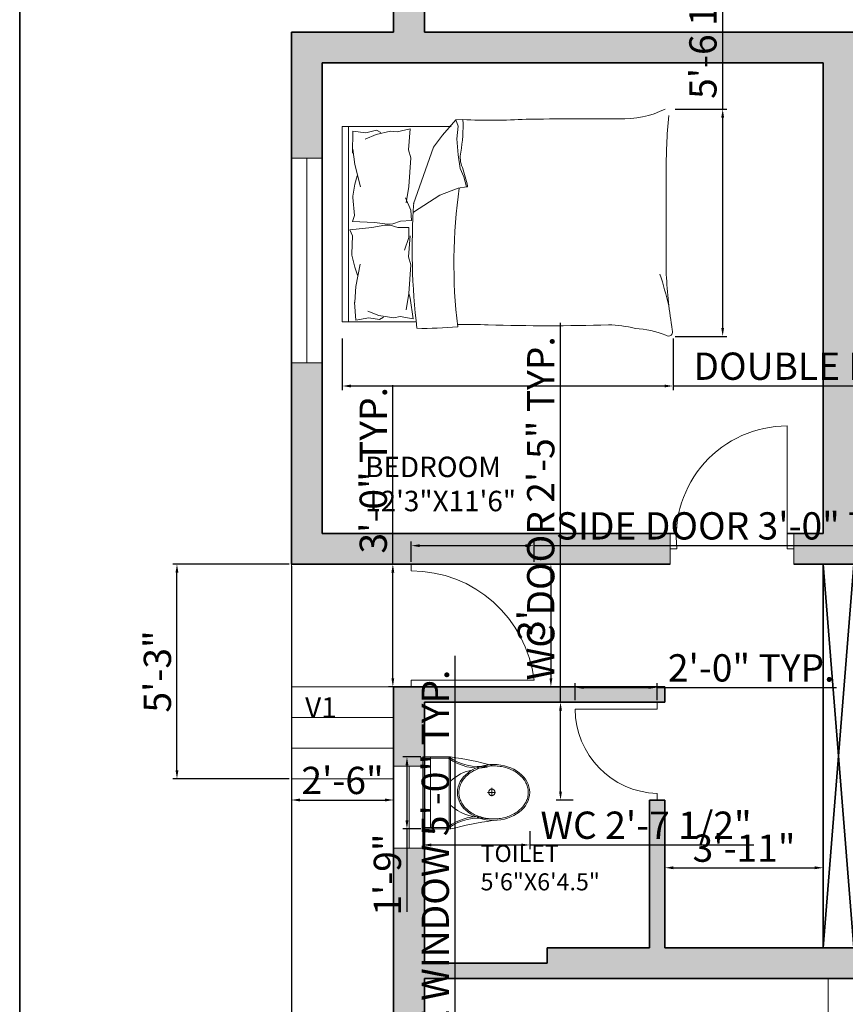
# Model space of a CAD drawing. Units: inches. Extents: x 2257 to 3678, y 834 to 1975.
# Tile 2 of 16: x 2257 to 2500, y 1155 to 1444. Entities that reach past the tile are written whole.
import ezdxf

# ---------------------------------------------------------------- set-up
doc = ezdxf.new("R2010")
doc.units = ezdxf.units.IN
for name, color, linetype, lineweight in [('A-ANNO-DIMS', 2, 'Continuous', 18), ('A-ANNO-TEXT', 7, 'Continuous', 18), ('A-ANNO-TTLB', 7, 'Continuous', 35), ('A-AREA-IDEN', 7, 'Continuous', 18), ('A-DOOR', 3, 'Continuous', 18), ('A-FLOR-CASE', 8, 'Continuous', 18), ('A-FLOR-FIXT', 9, 'Continuous', 18), ('A-FLOR-STRS', 7, 'Continuous', 18), ('A-FURN', 8, 'Continuous', 18), ('A-GLAZ', 4, 'Continuous', 18), ('A-WALL', 7, 'Continuous', 35)]:
    doc.layers.add(name, color=color, linetype=linetype, lineweight=lineweight)
doc.layers.add('A-WALL-PATT', color=251, linetype='Continuous', lineweight=13, true_color=0x636466)
doc.styles.get("Standard").update_dxf_attribs({"font": 'arial.ttf'})
doc.dimstyles.new('ISO-25', dxfattribs={"dimtxt": 8, "dimasz": 2.5, "dimexe": 1.25, "dimexo": 0.625, "dimtad": 1, "dimdec": 0, "dimlunit": 3, "dimtxsty": 'Standard', "dimcen": 2.5, "dimadec": 0, "dimazin": 0, "dimtfac": 1, "dimtdec": 0, "dimtmove": 0, "dimatfit": 3, "dimfxl": 1, "dimarcsym": 0})

# ---------------------------------------------------------------- blocks, each defined once
blk = doc.blocks.new('*D4')
at = {"layer": 'A-ANNO-DIMS', "color": 0, "lineweight": -2, "transparency": 16777216}
for p, q in [((2407.1, 1284.58), (2414.41, 1284.58)), ((2413.16, 1282.08), (2413.16, 1251.08)), ((2407.1, 1248.58), (2414.41, 1248.58))]:
    blk.add_line(p, q, dxfattribs=at)
at = {"layer": 'A-ANNO-DIMS', "color": 0, "transparency": 16777216}
for points in [[(2412.75, 1282.08), (2413.58, 1282.08), (2413.16, 1284.58)], [(2412.75, 1251.08), (2413.58, 1251.08), (2413.16, 1248.58)]]:
    blk.add_solid(points, dxfattribs=at)
at = {"layer": 'Defpoints', "color": 0, "transparency": 16777216}
for p in [(2406.47, 1284.58), (2406.47, 1248.58), (2413.16, 1248.58)]:
    blk.add_point(p, dxfattribs=at)
at = {"layer": 'A-ANNO-DIMS', "color": 0, "transparency": 16777216, "insert": (2408.45, 1266.58), "char_height": 8, "attachment_point": 5, "rotation": 90}
blk.add_mtext("3'", dxfattribs=at)
blk = doc.blocks.new('*D5')
at = {"layer": 'A-ANNO-DIMS', "color": 0, "lineweight": -2, "transparency": 16777216}
for p, q in [((2446.55, 1196.14), (2446.55, 1196.77)), ((2449.05, 1195.52), (2490.55, 1195.52)), ((2493.05, 1196.14), (2493.05, 1196.77))]:
    blk.add_line(p, q, dxfattribs=at)
at = {"layer": 'A-ANNO-DIMS', "color": 0, "transparency": 16777216}
for points in [[(2449.05, 1195.94), (2449.05, 1195.1), (2446.55, 1195.52)], [(2490.55, 1195.94), (2490.55, 1195.1), (2493.05, 1195.52)]]:
    blk.add_solid(points, dxfattribs=at)
at = {"layer": 'Defpoints', "color": 0, "transparency": 16777216}
for p in [(2446.55, 1195.52), (2493.05, 1195.52), (2493.05, 1195.52)]:
    blk.add_point(p, dxfattribs=at)
at = {"layer": 'A-ANNO-DIMS', "color": 0, "transparency": 16777216, "insert": (2469.8, 1200.23), "char_height": 8, "attachment_point": 5}
blk.add_mtext('3\'-11"', dxfattribs=at)
blk = doc.blocks.new('*D6')
at = {"layer": 'A-ANNO-DIMS', "color": 0, "lineweight": -2, "transparency": 16777216}
for p, q in [((2337.05, 1220.95), (2337.05, 1214.14)), ((2367.05, 1220.95), (2367.05, 1214.14)), ((2339.55, 1215.39), (2364.55, 1215.39))]:
    blk.add_line(p, q, dxfattribs=at)
at = {"layer": 'A-ANNO-DIMS', "color": 0, "transparency": 16777216}
for points in [[(2339.55, 1215.8), (2339.55, 1214.97), (2337.05, 1215.39)], [(2364.55, 1215.8), (2364.55, 1214.97), (2367.05, 1215.39)]]:
    blk.add_solid(points, dxfattribs=at)
at = {"layer": 'Defpoints', "color": 0, "transparency": 16777216}
for p in [(2337.05, 1221.58), (2367.05, 1221.58), (2367.05, 1215.39)]:
    blk.add_point(p, dxfattribs=at)
at = {"layer": 'A-ANNO-DIMS', "color": 0, "transparency": 16777216, "insert": (2352.05, 1220.09), "char_height": 8, "attachment_point": 5}
blk.add_mtext('2\'-6"', dxfattribs=at)
blk = doc.blocks.new('A$C31115884')
for p, q in [((283.1, 497.7), (223.4, 497.7)), ((257.5, 466.4), (257.5, 523.2)), ((0, 200), (0, 0)), ((520, 200), (0, 200)), ((10, 190), (10, 10)), ((510, 190), (10, 190)), ((510, 10), (510, 190)), ((520, 0), (520, 200)), ((510, 54.5), (0, 54.5)), ((10, 10), (510, 10)), ((0, 0), (520, 0))]:
    blk.add_line(p, q)
blk.add_circle((255.6, 496.4), 23.6)
for centre, radius, start, end in [((2777.7, -204.6), 2807, 165.4549, 171.71327), ((3237, 905), 2807, 188.28673, 194.5451), ((-294.5, 403.3), 364.7, 324.20913, 9.34987), ((-294.5, 403.3), 374.7, 324.20913, 9.34987), ((805.8, 403.3), 364.7, 170.65013, 215.79087), ((139.5, 406.2), 293.5, 315.84364, 2.65635), ((805.8, 403.3), 374.7, 179.20365, 215.79087), ((383.6, 406.2), 293.5, 190.27735, 224.15636)]:
    blk.add_arc(centre, radius, start, end)
blk.add_ellipse((256.2, 509.9), major_axis=(0, -260.7), ratio=0.772727)
blk.add_open_spline([(256.2, 259.2), (263.1, 259.2), (270, 259.7), (287.8, 262.3), (298.7, 265.1), (319.9, 273.1), (330.2, 278.4), (350.1, 291.1), (359.7, 298.7), (377.7, 315.9), (386.2, 325.5), (401.7, 346.6), (408.8, 358.1), (421.3, 382.5), (426.8, 395.5), (435.9, 422.4), (439.5, 436.4), (444.8, 465.1), (446.5, 479.7), (447.9, 509.2), (447.6, 524), (445, 553.3), (442.7, 567.8), (436.3, 596), (432.1, 609.7), (421.9, 636), (416, 648.6), (402.5, 672.1), (395, 683), (378.6, 703), (369.8, 712.1), (351.1, 728), (341.3, 734.8), (320.9, 746.2), (310.4, 750.7), (288.9, 757.3), (278, 759.4), (256, 761), (245, 760.6), (223.1, 757.2), (212.3, 754.3), (191.1, 746.1), (180.8, 740.7), (160.9, 727.8), (151.4, 720.1), (133.5, 702.7), (125.1, 693), (109.6, 671.7), (102.6, 660.2), (90.2, 635.7), (84.9, 622.7), (76, 595.6), (72.4, 581.6), (67.2, 552.9), (65.6, 538.2), (64.4, 508.8), (64.8, 494), (67.5, 464.7), (69.9, 450.2), (76.6, 422), (80.8, 408.3), (91.1, 382.2), (97.2, 369.7), (110.8, 346.3), (118.4, 335.4), (134.8, 315.6), (143.7, 306.7), (162.4, 290.9), (172.3, 284.2), (192.8, 273), (203.3, 268.6), (224.8, 262.2), (235.8, 260.2), (249.9, 259.3), (253, 259.2), (256.2, 259.2)], degree=3, knots=[0, 0, 0, 0, 0.110105, 0.110105, 0.285049, 0.285049, 0.459994, 0.459994, 0.634938, 0.634938, 0.809882, 0.809882, 0.984827, 0.984827, 1.159771, 1.159771, 1.334715, 1.334715, 1.50966, 1.50966, 1.684604, 1.684604, 1.859549, 1.859549, 2.034493, 2.034493, 2.209437, 2.209437, 2.384382, 2.384382, 2.559326, 2.559326, 2.73427, 2.73427, 2.909215, 2.909215, 3.084159, 3.084159, 3.259103, 3.259103, 3.434048, 3.434048, 3.608992, 3.608992, 3.783936, 3.783936, 3.958881, 3.958881, 4.133825, 4.133825, 4.30877, 4.30877, 4.483714, 4.483714, 4.658658, 4.658658, 4.833603, 4.833603, 5.008547, 5.008547, 5.183491, 5.183491, 5.358436, 5.358436, 5.53338, 5.53338, 5.708324, 5.708324, 5.883269, 5.883269, 6.058213, 6.058213, 6.233158, 6.233158, 6.283185, 6.283185, 6.283185, 6.283185])
blk = doc.blocks.new('BED-DOUBLE-PLAN')
for p, q in [((0, 61.46), (31.9, 61.46)), ((0, 4.17), (0, 61.46)), ((1.84, 4.17), (1.84, 61.46)), ((19.87, 60.78), (16.11, 59.85)), ((19.38, 54.63), (19.87, 60.78)), ((33.26, 63.38), (29.37, 58.94)), ((35.36, 63.48), (33.26, 63.38, 4.64)), ((34.01, 61.54), (33.26, 63.38)), ((33.63, 57.82), (34.01, 61.54)), ((3.07, 60.08), (2.95, 53.6)), ((3.07, 60.08), (6.92, 59.62)), ((9.9, 59.11), (6.69, 57.7)), ((6.92, 59.62), (10, 60.34)), ((14.18, 60.08), (9.9, 59.11)), ((10, 60.34), (11.25, 59.72)), ((16.11, 59.85), (14.18, 60.08)), ((29.37, 58.94), (26.77, 55.41)), ((34.01, 53.18), (33.63, 57.82)), ((26.77, 55.41), (24.36, 48.73)), ((2.95, 53.6), (3.05, 54.8)), ((3.05, 54.8), (3.68, 50.25)), ((20.05, 52.28), (19.38, 54.63)), ((19.54, 43.87), (20.05, 52.28)), ((34.56, 49.1), (34.01, 53.18)), ((3.68, 50.25), (5.3, 43.75)), ((35.68, 46.68), (34.56, 49.1)), ((4.4, 47), (3.69, 44.52)), ((24.36, 48.73), (20.84, 38.73)), ((36.42, 43.71), (35.68, 46.68)), ((95, 18.06), (95, 47.57)), ((3.69, 44.52), (3.04, 41.01)), ((18.74, 39.04), (19.54, 43.87)), ((28.62, 41.3), (34.01, 43.34)), ((34.01, 43.34), (36.42, 43.71)), ((3.04, 41.01), (3.07, 40.62)), ((3.07, 40.62), (3.57, 35.31)), ((20.07, 36.86), (18.53, 40.55)), ((20.84, 36.28), (28.62, 41.3)), ((3.57, 35.31), (2.99, 33.54)), ((20.25, 33.92), (20.07, 36.86)), ((2.24, 31.15), (8.66, 31.84)), ((2.99, 33.54), (9.43, 33.25)), ((8.66, 31.84), (12.47, 32.54)), ((9.43, 33.25), (13.28, 32.79)), ((12.47, 32.54), (14.03, 32.54)), ((13.28, 32.79), (14.84, 32.89)), ((14.03, 32.54), (16.28, 31.84)), ((14.84, 32.89), (17.04, 33.72)), ((16.28, 31.84), (19.5, 31.84)), ((17.04, 33.72), (20.25, 33.92)), ((19.5, 31.84), (19.5, 28.9)), ((2.94, 29.42), (2.24, 31.15)), ((2.76, 24.09), (2.94, 29.42)), ((19.5, 28.9), (18.19, 25.13)), ((19.38, 23.24), (19.87, 29.39)), ((2.76, 23.7), (2.76, 24.09)), ((3.63, 20.23), (2.76, 23.7)), ((20.05, 20.89), (19.38, 23.24)), ((4.5, 17.81), (3.63, 20.23)), ((3.98, 14.52), (5.19, 21.1)), ((19.54, 12.48), (20.05, 20.89)), ((3.63, 9.93), (3.98, 14.52)), ((18.74, 7.65), (19.54, 12.48)), ((19.54, 12.48), (19.92, 11.13)), ((3.61, 9.81), (3.63, 9.93)), ((4, 4.67), (3.61, 9.81)), ((19.92, 11.13), (20.79, 5.02)), ((10.74, 6.06), (7.44, 7.27)), ((15.07, 5.36), (10.74, 6.06)), ((21.71, 4.17), (0, 4.17)), ((3.98, 4.67), (7.79, 5.36)), ((7.79, 5.36), (10.91, 4.84)), ((10.91, 4.84), (12.12, 5.54)), ((16.98, 5.71), (15.07, 5.36)), ((20.79, 5.02), (16.98, 5.71))]:
    blk.add_line(p, q)
for centre, radius, start, end in [((82.32, 91.3), 27.65, 267.4714, 296.4681), ((43.54, 218.51), 155.25, 266.9791, 273.8365), ((81.31, -5405.34), 5469.02, 90.00217, 90.28689), ((254.49, 49.33), 159.5, 174.4998, 180.6351), ((-7.98, 61.53), 43.38, 349.8763, 2.5657), ((42.04, 52.44), 7.46, 168.6608, 203.7384), ((1.78, 37.35), 35.55, 10.6617, 19.8806), ((187.4, 21.29), 154.68, 171.7845, 186.9006), ((36.49, 43.92), 0.221, 250.2464, 1.1377), ((218.26, 25.61), 197.77, 176.0865, 186.7821), ((-28.43, -20.65), 127.63, 13.3832, 17.7053), ((240.78, 25.69), 145.97, 182.9958, 189.4091), ((37.37, -200.58), 203.94, 88.4762, 91.0082), ((60.68, 581.23), 578.22, 268.22771, 271.71854), ((77.34, -32.25), 35.53, 76.0648, 88.9113), ((24.09, 102.1), 99.87, 268.7218, 275.604), ((84.25, -25.97), 28.25, 67.9751, 86.652), ((95.57, 1.3), 1.31, 236.1736, 23.4781)]:
    blk.add_arc(centre, radius, start, end)
blk = doc.blocks.new('WIN-60')
for p, q in [((0, 9), (0, 0)), ((60, 4.5), (60, 9)), ((60, 9), (60, 0)), ((0, 0), (0, 4.5)), ((0, 4.5), (60, 4.5))]:
    blk.add_line(p, q)
blk = doc.blocks.new('WIN-24')
for p, q in [((0, 9), (0, 0)), ((24, 4.5), (24, 9)), ((24, 9), (24, 0)), ((0, 0), (0, 4.5)), ((0, 4.5), (24, 4.5))]:
    blk.add_line(p, q)
blk = doc.blocks.new('DOOR-WC')
for p, q in [((24, 26.75), (0, 26.75)), ((24, 28.75), (24, 26.75)), ((24, 26.75), (24, 28.75)), ((24, 0), (24, 2)), ((24, 0), (24, 2))]:
    blk.add_line(p, q)
blk.add_arc((24.77, 26.75), 24.77, 180, 268.2255)
blk = doc.blocks.new('DOOR-BEDROOM-WEST')
for p, q in [((34.29, 4.5), (34.29, 40.5)), ((0, 9), (0, 0)), ((36.29, 9), (36.29, 0)), ((0, 0), (0, 4.5)), ((0, 4.5), (2, 4.5)), ((36.29, 4.5), (34.29, 4.5)), ((36.29, 0), (36.29, 4.5)), ((0, 0), (0, 0))]:
    blk.add_line(p, q)
blk.add_arc((34.29, 8.02), 32.48, 90, 186.2235)
blk = doc.blocks.new('DOOR-SIDE-ENTRY')
for p, q in [((0, 36), (0, 34)), ((0, 0), (0, 2)), ((0, 2), (24, 2)), ((24, 2), (36, 2))]:
    blk.add_line(p, q)
blk.add_arc((0, -2.25), 36.25, 6.7329, 90)
blk = doc.blocks.new('STEPS-SIDE-ENTRY')
for p, q in [((0, 69.18), (0, 3.09)), ((30, 30.09), (0, 30.09)), ((30, 18), (30, 27)), ((0, 12.09), (0, 21.09)), ((0, 21.09), (30, 21.09)), ((30, 12.09), (0, 12.09)), ((30, 0), (30, 9)), ((0, 3.09), (30, 3.09))]:
    blk.add_line(p, q)
blk = doc.blocks.new('*D48')
at = {"layer": 'A-ANNO-DIMS', "color": 0, "lineweight": -2, "transparency": 16777216}
for p, q in [((2351.99, 1350.73), (2351.99, 1335.55)), ((2448.99, 1350.73), (2448.99, 1335.55)), ((2354.49, 1336.8), (2446.49, 1336.8)), ((2448.99, 1336.8), (2576.25, 1336.8))]:
    blk.add_line(p, q, dxfattribs=at)
at = {"layer": 'A-ANNO-DIMS', "color": 0, "transparency": 16777216}
for points in [[(2354.49, 1337.22), (2354.49, 1336.39), (2351.99, 1336.8)], [(2446.49, 1337.22), (2446.49, 1336.39), (2448.99, 1336.8)]]:
    blk.add_solid(points, dxfattribs=at)
at = {"layer": 'Defpoints', "color": 0, "transparency": 16777216}
for p in [(2351.99, 1351.35), (2448.99, 1351.35), (2448.99, 1336.8)]:
    blk.add_point(p, dxfattribs=at)
at = {"layer": 'A-ANNO-DIMS', "color": 0, "transparency": 16777216, "insert": (2513.87, 1341.57), "char_height": 8, "attachment_point": 5}
blk.add_mtext('DOUBLE BED 8\'-1" TYP.', dxfattribs=at)
blk = doc.blocks.new('*D49')
at = {"layer": 'A-ANNO-DIMS', "color": 0, "lineweight": -2, "transparency": 16777216}
for p, q in [((2463.54, 1418), (2463.54, 1489.16)), ((2449.61, 1418), (2464.79, 1418)), ((2463.54, 1353.85), (2463.54, 1415.5)), ((2449.61, 1351.35), (2464.79, 1351.35))]:
    blk.add_line(p, q, dxfattribs=at)
at = {"layer": 'A-ANNO-DIMS', "color": 0, "transparency": 16777216}
for points in [[(2463.12, 1415.5), (2463.95, 1415.5), (2463.54, 1418)], [(2463.12, 1353.85), (2463.95, 1353.85), (2463.54, 1351.35)]]:
    blk.add_solid(points, dxfattribs=at)
at = {"layer": 'Defpoints', "color": 0, "transparency": 16777216}
for p in [(2448.99, 1418), (2463.54, 1418), (2448.99, 1351.35)]:
    blk.add_point(p, dxfattribs=at)
at = {"layer": 'A-ANNO-DIMS', "color": 0, "transparency": 16777216, "insert": (2458.78, 1454.83), "char_height": 8, "attachment_point": 5, "rotation": 90}
blk.add_mtext('5\'-6 1/2" TYP.', dxfattribs=at)
blk = doc.blocks.new('*D52')
at = {"layer": 'A-ANNO-DIMS', "color": 0, "lineweight": -2, "transparency": 16777216}
for p, q in [((2375.64, 1206.27), (2375.64, 1200.95)), ((2406.95, 1206.27), (2406.95, 1200.95)), ((2378.14, 1202.2), (2404.45, 1202.2)), ((2406.95, 1202.2), (2472.66, 1202.2))]:
    blk.add_line(p, q, dxfattribs=at)
at = {"layer": 'A-ANNO-DIMS', "color": 0, "transparency": 16777216}
for points in [[(2378.14, 1202.62), (2378.14, 1201.78), (2375.64, 1202.2)], [(2404.45, 1202.62), (2404.45, 1201.78), (2406.95, 1202.2)]]:
    blk.add_solid(points, dxfattribs=at)
at = {"layer": 'Defpoints', "color": 0, "transparency": 16777216}
for p in [(2375.64, 1206.89), (2406.95, 1206.89), (2406.95, 1202.2)]:
    blk.add_point(p, dxfattribs=at)
at = {"layer": 'A-ANNO-DIMS', "color": 0, "transparency": 16777216, "insert": (2441.06, 1206.96), "char_height": 8, "attachment_point": 5}
blk.add_mtext('WC 2\'-7 1/2"', dxfattribs=at)
blk = doc.blocks.new('*D53')
at = {"layer": 'A-ANNO-DIMS', "color": 0, "lineweight": -2, "transparency": 16777216}
for p, q in [((2375.02, 1228.02), (2369.7, 1228.02)), ((2370.95, 1225.52), (2370.95, 1209.39)), ((2375.02, 1206.89), (2369.7, 1206.89)), ((2370.95, 1206.89), (2370.95, 1182.63))]:
    blk.add_line(p, q, dxfattribs=at)
at = {"layer": 'A-ANNO-DIMS', "color": 0, "transparency": 16777216}
for points in [[(2370.53, 1225.52), (2371.37, 1225.52), (2370.95, 1228.02)], [(2370.53, 1209.39), (2371.37, 1209.39), (2370.95, 1206.89)]]:
    blk.add_solid(points, dxfattribs=at)
at = {"layer": 'Defpoints', "color": 0, "transparency": 16777216}
for p in [(2375.64, 1228.02), (2370.95, 1206.89), (2375.64, 1206.89)]:
    blk.add_point(p, dxfattribs=at)
at = {"layer": 'A-ANNO-DIMS', "color": 0, "transparency": 16777216, "insert": (2366.24, 1193.51), "char_height": 8, "attachment_point": 5, "rotation": 90}
blk.add_mtext('1\'-9"', dxfattribs=at)
blk = doc.blocks.new('*D58')
at = {"layer": 'A-ANNO-DIMS', "color": 0, "lineweight": -2, "transparency": 16777216}
for p, q in [((2385.05, 1123.86), (2385.05, 1257.67)), ((2376.68, 1123.86), (2386.3, 1123.86)), ((2385.05, 1066.36), (2385.05, 1121.36)), ((2376.68, 1063.86), (2386.3, 1063.86))]:
    blk.add_line(p, q, dxfattribs=at)
at = {"layer": 'A-ANNO-DIMS', "color": 0, "transparency": 16777216}
for points in [[(2384.63, 1121.36), (2385.47, 1121.36), (2385.05, 1123.86)], [(2384.63, 1066.36), (2385.47, 1066.36), (2385.05, 1063.86)]]:
    blk.add_solid(points, dxfattribs=at)
at = {"layer": 'Defpoints', "color": 0, "transparency": 16777216}
for p in [(2376.05, 1123.86), (2385.05, 1123.86), (2376.05, 1063.86)]:
    blk.add_point(p, dxfattribs=at)
at = {"layer": 'A-ANNO-DIMS', "color": 0, "transparency": 16777216, "insert": (2380.29, 1192.01), "char_height": 8, "attachment_point": 5, "rotation": 90}
blk.add_mtext('SIDE WINDOW 5\'-0" TYP.', dxfattribs=at)
blk = doc.blocks.new('*D72')
at = {"layer": 'A-ANNO-DIMS', "color": 0, "lineweight": -2, "transparency": 16777216}
for p, q in [((2415.99, 1244.08), (2415.99, 1355.28)), ((2419.68, 1244.08), (2414.74, 1244.08)), ((2415.99, 1217.82), (2415.99, 1241.58)), ((2419.68, 1215.32), (2414.74, 1215.32))]:
    blk.add_line(p, q, dxfattribs=at)
at = {"layer": 'A-ANNO-DIMS', "color": 0, "transparency": 16777216}
for points in [[(2415.57, 1241.58), (2416.4, 1241.58), (2415.99, 1244.08)], [(2415.57, 1217.82), (2416.4, 1217.82), (2415.99, 1215.32)]]:
    blk.add_solid(points, dxfattribs=at)
at = {"layer": 'Defpoints', "color": 0, "transparency": 16777216}
for p in [(2415.99, 1244.08), (2420.3, 1244.08), (2420.3, 1215.32)]:
    blk.add_point(p, dxfattribs=at)
at = {"layer": 'A-ANNO-DIMS', "color": 0, "transparency": 16777216, "insert": (2411.22, 1300.93), "char_height": 8, "attachment_point": 5, "rotation": 90}
blk.add_mtext('WC DOOR 2\'-5" TYP.', dxfattribs=at)
blk = doc.blocks.new('*D73')
at = {"layer": 'A-ANNO-DIMS', "color": 0, "lineweight": -2, "transparency": 16777216}
for p, q in [((2420.3, 1244.7), (2420.3, 1249.64)), ((2422.8, 1248.39), (2441.8, 1248.39)), ((2444.3, 1244.7), (2444.3, 1249.64)), ((2444.3, 1248.39), (2496.95, 1248.39))]:
    blk.add_line(p, q, dxfattribs=at)
at = {"layer": 'A-ANNO-DIMS', "color": 0, "transparency": 16777216}
for points in [[(2422.8, 1248.81), (2422.8, 1247.97), (2420.3, 1248.39)], [(2441.8, 1248.81), (2441.8, 1247.97), (2444.3, 1248.39)]]:
    blk.add_solid(points, dxfattribs=at)
at = {"layer": 'Defpoints', "color": 0, "transparency": 16777216}
for p in [(2444.3, 1248.39), (2420.3, 1244.08), (2444.3, 1244.08)]:
    blk.add_point(p, dxfattribs=at)
at = {"layer": 'A-ANNO-DIMS', "color": 0, "transparency": 16777216, "insert": (2471.88, 1253.1), "char_height": 8, "attachment_point": 5}
blk.add_mtext('2\'-0" TYP.', dxfattribs=at)
blk = doc.blocks.new('*D80')
at = {"layer": 'A-ANNO-DIMS', "color": 0, "lineweight": -2, "transparency": 16777216}
for p, q in [((2372.21, 1285.2), (2372.21, 1291.23)), ((2408.21, 1285.2), (2408.21, 1291.23)), ((2374.71, 1289.98), (2405.71, 1289.98)), ((2408.21, 1289.98), (2526.51, 1289.98))]:
    blk.add_line(p, q, dxfattribs=at)
at = {"layer": 'A-ANNO-DIMS', "color": 0, "transparency": 16777216}
for points in [[(2374.71, 1290.39), (2374.71, 1289.56), (2372.21, 1289.98)], [(2405.71, 1290.39), (2405.71, 1289.56), (2408.21, 1289.98)]]:
    blk.add_solid(points, dxfattribs=at)
at = {"layer": 'Defpoints', "color": 0, "transparency": 16777216}
for p in [(2408.21, 1289.98), (2372.21, 1284.58), (2408.21, 1284.58)]:
    blk.add_point(p, dxfattribs=at)
at = {"layer": 'A-ANNO-DIMS', "color": 0, "transparency": 16777216, "insert": (2468.61, 1294.74), "char_height": 8, "attachment_point": 5}
blk.add_mtext('SIDE DOOR 3\'-0" TYP.', dxfattribs=at)
blk = doc.blocks.new('*D81')
at = {"layer": 'A-ANNO-DIMS', "color": 0, "lineweight": -2, "transparency": 16777216}
for p, q in [((2366.81, 1284.58), (2366.81, 1337.09)), ((2371.58, 1284.58), (2365.56, 1284.58)), ((2366.81, 1251.08), (2366.81, 1282.08)), ((2371.58, 1248.58), (2365.56, 1248.58))]:
    blk.add_line(p, q, dxfattribs=at)
at = {"layer": 'A-ANNO-DIMS', "color": 0, "transparency": 16777216}
for points in [[(2366.39, 1282.08), (2367.22, 1282.08), (2366.81, 1284.58)], [(2366.39, 1251.08), (2367.22, 1251.08), (2366.81, 1248.58)]]:
    blk.add_solid(points, dxfattribs=at)
at = {"layer": 'Defpoints', "color": 0, "transparency": 16777216}
for p in [(2366.81, 1284.58), (2372.21, 1284.58), (2372.21, 1248.58)]:
    blk.add_point(p, dxfattribs=at)
at = {"layer": 'A-ANNO-DIMS', "color": 0, "transparency": 16777216, "insert": (2362.1, 1312.08), "char_height": 8, "attachment_point": 5, "rotation": 90}
blk.add_mtext('3\'-0" TYP.', dxfattribs=at)
blk = doc.blocks.new('*D96')
at = {"layer": 'A-ANNO-DIMS', "color": 0, "lineweight": -2, "transparency": 16777216}
for p, q in [((2337.05, 1283.95), (2337.05, 894.3)), ((2883.34, 1168.45), (2883.34, 894.3)), ((2339.55, 895.55), (2880.84, 895.55))]:
    blk.add_line(p, q, dxfattribs=at)
at = {"layer": 'A-ANNO-DIMS', "color": 0, "transparency": 16777216}
for points in [[(2339.55, 895.97), (2339.55, 895.14), (2337.05, 895.55)], [(2880.84, 895.97), (2880.84, 895.14), (2883.34, 895.55)]]:
    blk.add_solid(points, dxfattribs=at)
at = {"layer": 'Defpoints', "color": 0, "transparency": 16777216}
for p in [(2337.05, 1284.58), (2883.34, 1169.08), (2883.34, 895.55)]:
    blk.add_point(p, dxfattribs=at)
at = {"layer": 'A-ANNO-DIMS', "color": 0, "transparency": 16777216, "insert": (2610.2, 900.31), "char_height": 8, "attachment_point": 5}
blk.add_mtext('45\'-6 1/2"', dxfattribs=at)
blk = doc.blocks.new('*D98')
at = {"layer": 'A-ANNO-DIMS', "color": 0, "lineweight": -2, "transparency": 16777216}
for p, q in [((2336.43, 1284.58), (2302.25, 1284.58)), ((2303.5, 1224.08), (2303.5, 1282.08)), ((2336.43, 1221.58), (2302.25, 1221.58))]:
    blk.add_line(p, q, dxfattribs=at)
at = {"layer": 'A-ANNO-DIMS', "color": 0, "transparency": 16777216}
for points in [[(2303.08, 1282.08), (2303.92, 1282.08), (2303.5, 1284.58)], [(2303.08, 1224.08), (2303.92, 1224.08), (2303.5, 1221.58)]]:
    blk.add_solid(points, dxfattribs=at)
at = {"layer": 'Defpoints', "color": 0, "transparency": 16777216}
for p in [(2303.5, 1284.58), (2337.05, 1284.58), (2337.05, 1221.58)]:
    blk.add_point(p, dxfattribs=at)
at = {"layer": 'A-ANNO-DIMS', "color": 0, "transparency": 16777216, "insert": (2298.79, 1253.08), "char_height": 8, "attachment_point": 5, "rotation": 90}
blk.add_mtext('5\'-3"', dxfattribs=at)

msp = doc.modelspace()

# ---------------------------------------------------------------- hatches: boundary and pattern name
at = {"layer": 'A-WALL-PATT'}
h = msp.add_hatch(color=256, dxfattribs=at)
h.dxf.hatch_style = 1
h.paths.add_polyline_path([(2736.02, 1589.08), (2736.02, 1593.58), (2691.05, 1593.58), (2648.2, 1593.58), (2648.2, 1584.58), (2691.05, 1584.58), (2691.05, 1485.58), (2700.05, 1485.58), (2700.05, 1584.58), (2736.02, 1584.58)])
h.paths.add_polyline_path([(2835.05, 1593.58), (2796.02, 1593.58), (2796.02, 1584.58), (2826.05, 1584.58), (2826.05, 1440.58), (2835.05, 1440.58)])
h.paths.add_polyline_path([(2865.05, 1440.58), (2826.05, 1440.58), (2700.05, 1440.58), (2691.05, 1440.58), (2691.05, 1431.58), (2691.05, 1284.58), (2700.05, 1284.58), (2700.05, 1431.58), (2826.05, 1431.58), (2856.05, 1431.58), (2856.05, 1395.2), (2865.05, 1395.2), (2865.05, 1431.58)])
h.paths.add_polyline_path([(2865.05, 1335.2), (2856.05, 1335.2), (2856.05, 1293.58), (2741.94, 1293.58), (2741.94, 1289.08), (2741.94, 1284.58), (2865.05, 1284.58)], flags=17)
h.paths.add_polyline_path([(2865.05, 1172.08), (2856.05, 1172.08), (2741.94, 1172.08), (2741.94, 1163.08), (2856.05, 1163.08), (2856.05, 1133.53), (2865.05, 1133.53)])
h.paths.add_polyline_path([(2865.05, 1073.53), (2856.05, 1073.53), (2856.05, 1019.08), (2795.28, 1019.08), (2795.28, 1010.08), (2865.05, 1010.08)])
h.paths.add_polyline_path([(2735.28, 1014.58), (2735.28, 1019.08), (2700.05, 1019.08), (2700.05, 1026.35), (2695.55, 1026.35), (2691.05, 1026.35), (2691.05, 1010.08), (2735.28, 1010.08)])
h.paths.add_polyline_path([(2700.05, 1163.08), (2700.05, 1172.08), (2691.05, 1172.08), (2685.7, 1172.08), (2685.7, 1163.08), (2691.05, 1163.08), (2691.05, 1058.19), (2700.05, 1058.19)])
h.paths.add_polyline_path([(2707.1, 1172.08), (2700.05, 1172.08), (2700.05, 1163.08), (2707.1, 1163.08)])
h.paths.add_polyline_path([(2685.7, 1172.08), (2678.22, 1172.08), (2678.22, 1163.08), (2685.7, 1163.08)])
h.paths.add_polyline_path([(2654.22, 1172.08), (2648.96, 1172.08), (2648.96, 1163.08), (2654.22, 1163.08), (2654.22, 1167.58)])
h.paths.add_polyline_path([(2553.05, 1163.08), (2558.66, 1163.08), (2558.66, 1172.08), (2544.05, 1172.08), (2544.05, 1163.08), (2544.05, 1058.19), (2553.05, 1058.19)])
h.paths.add_polyline_path([(2568.8, 1167.58), (2568.8, 1172.08), (2558.66, 1172.08), (2558.66, 1163.08), (2568.8, 1163.08)])
h.paths.add_polyline_path([(2596.82, 1172.08), (2592.8, 1172.08), (2592.8, 1163.08), (2596.82, 1163.08)])
h.paths.add_polyline_path([(2553.05, 1019.08), (2553.05, 1026.35), (2548.55, 1026.35), (2544.05, 1026.35), (2544.05, 1019.08), (2476.8, 1019.08), (2476.8, 1010.08), (2553.05, 1010.08)])
h.paths.add_polyline_path([(2376.05, 1163.08), (2502.05, 1163.08), (2502.05, 1172.08), (2446.55, 1172.08), (2446.55, 1195.52), (2446.55, 1215.32), (2442.05, 1215.32), (2442.05, 1195.52), (2442.05, 1172.08), (2412.05, 1172.08), (2412.05, 1167.58), (2376.05, 1167.58), (2376.05, 1172.08), (2376.05, 1201.28), (2367.05, 1201.28), (2367.05, 1172.08), (2367.05, 1123.86), (2376.05, 1123.86)])
h.paths.add_polyline_path([(2577.05, 1440.58), (2376.05, 1440.58), (2376.05, 1485.89), (2367.05, 1485.89), (2367.05, 1440.58), (2337.05, 1440.58), (2337.05, 1403.59), (2346.05, 1403.59), (2346.05, 1431.58), (2493.05, 1431.58), (2493.05, 1293.58), (2484.41, 1293.58), (2484.41, 1284.58), (2502.05, 1284.58), (2502.05, 1431.58), (2577.05, 1431.58)])
h.paths.add_polyline_path([(2346.05, 1343.59), (2337.05, 1343.59), (2337.05, 1284.58), (2448.12, 1284.58), (2448.12, 1289.08), (2448.12, 1293.58), (2346.05, 1293.58)], flags=17)
h.paths.add_polyline_path([(2376.05, 1244.08), (2446.55, 1244.08), (2446.55, 1248.58), (2367.05, 1248.58), (2367.05, 1225.28), (2375.64, 1225.28), (2375.64, 1228.02), (2376.05, 1228.02)])
h.paths.add_polyline_path([(2588.2, 1589.08), (2588.2, 1593.58), (2468.1, 1593.58), (2468.1, 1584.58), (2544.05, 1584.58), (2544.05, 1541.08), (2568.05, 1541.08), (2568.05, 1490.08), (2544.05, 1490.08), (2544.05, 1485.58), (2577.05, 1485.58), (2577.05, 1545.58), (2553.05, 1545.58), (2553.05, 1584.58), (2588.2, 1584.58)])
h.paths.add_polyline_path([(2376.05, 1584.58), (2408.1, 1584.58), (2408.1, 1589.08), (2408.1, 1593.58), (2367.05, 1593.58), (2367.05, 1545.89), (2376.05, 1545.89)])
h.paths.add_polyline_path([(2376.05, 1063.86), (2367.05, 1063.86), (2367.05, 1019.08), (2367.05, 1010.08), (2416.8, 1010.08), (2416.8, 1014.58), (2416.8, 1019.08), (2376.05, 1019.08)])

# ---------------------------------------------------------------- linework, layer by layer
at = {"layer": 'A-ANNO-TTLB'}
msp.add_lwpolyline([(2257.38, 1974.9), (3677.96, 1974.9), (3677.96, 849.42), (2257.38, 849.42)], close=True, dxfattribs=at)
at = {"layer": 'A-FLOR-CASE'}
msp.add_line((2494.46, 1139.28), (2494.46, 1163.08), dxfattribs=at)
at = {"layer": 'A-GLAZ'}
for p, q in [((2337.05, 1403.59), (2337.05, 1403.59)), ((2367.05, 1225.28), (2367.05, 1225.28))]:
    msp.add_line(p, q, dxfattribs=at)
at = {"layer": 'A-WALL'}
for p, q in [((2367.05, 1593.58), (2367.05, 1440.58)), ((2376.05, 1584.58), (2376.05, 1440.58)), ((2337.05, 1440.58), (2367.05, 1440.58)), ((2337.05, 1440.58), (2337.05, 1284.58)), ((2376.05, 1440.58), (2691.05, 1440.58)), ((2346.05, 1431.58), (2493.05, 1431.58)), ((2346.05, 1431.58), (2346.05, 1293.58)), ((2493.05, 1431.58), (2493.05, 1293.58)), ((2346.05, 1293.58), (2449.94, 1293.58)), ((2482.41, 1293.58), (2493.05, 1293.58)), ((2337.05, 1284.58), (2448.12, 1284.58)), ((2484.41, 1284.58), (2502.05, 1284.58)), ((2493.05, 1284.58), (2493.05, 1172.08)), ((2493.05, 1284.58), (2502.05, 1172.08)), ((2493.05, 1172.08), (2502.05, 1284.58)), ((2367.05, 1248.58), (2446.55, 1248.58)), ((2367.05, 1172.08), (2367.05, 1248.58)), ((2446.55, 1244.08), (2446.55, 1248.58)), ((2376.05, 1244.08), (2446.55, 1244.08)), ((2376.05, 1172.08), (2376.05, 1244.08)), ((2442.05, 1195.52), (2442.05, 1215.32)), ((2442.05, 1215.32), (2446.55, 1215.32)), ((2446.55, 1215.32), (2446.55, 1195.52)), ((2442.05, 1172.08), (2442.05, 1195.52)), ((2446.55, 1195.52), (2446.55, 1172.08)), ((2367.05, 1172.08), (2367.05, 1010.08)), ((2376.05, 1172.08), (2376.05, 1167.58)), ((2412.05, 1172.08), (2442.05, 1172.08)), ((2412.05, 1167.58), (2412.05, 1172.08)), ((2446.55, 1172.08), (2598.82, 1172.08)), ((2376.05, 1167.58), (2412.05, 1167.58)), ((2367.05, 1163.08), (2367.05, 1019.08)), ((2376.05, 1163.08), (2544.05, 1163.08)), ((2376.05, 1163.08), (2376.05, 1019.08)), ((2446.55, 1163.08), (2442.05, 1163.08))]:
    msp.add_line(p, q, dxfattribs=at)

# ---------------------------------------------------------------- block references
at = {"layer": 'A-DOOR'}
for name, p in [('DOOR-BEDROOM-WEST', (2448.12, 1284.58)), ('DOOR-SIDE-ENTRY', (2372.21, 1248.58)), ('DOOR-WC', (2420.3, 1215.32))]:
    msp.add_blockref(name, p, dxfattribs=at)
at = {"layer": 'A-FLOR-FIXT', "xscale": 0.0406268506401408, "yscale": 0.0406268506401408, "zscale": 0.0406268506401408, "rotation": 269.9999999999999}
msp.add_blockref('A$C31115884', (2375.64, 1228.02), dxfattribs=at)
at = {"layer": 'A-FLOR-STRS'}
msp.add_blockref('STEPS-SIDE-ENTRY', (2337.05, 1218.48), dxfattribs=at)
at = {"layer": 'A-FURN'}
msp.add_blockref('BED-DOUBLE-PLAN', (2351.99, 1351.46), dxfattribs=at)
at = {"layer": 'A-GLAZ', "extrusion": (0, 0, -1), "zscale": -1}
for name, p, rotation in [('WIN-60', (-2346.05, 1403.59), 270.0000000000001), ('WIN-24', (-2376.05, 1225.28), 269.9999999999958)]:
    msp.add_blockref(name, p, dxfattribs=dict(at, rotation=rotation))

# ---------------------------------------------------------------- texts
at = {"layer": 'A-ANNO-TEXT', "insert": (2341.08, 1245.53), "char_height": 6, "attachment_point": 1}
msp.add_mtext_dynamic_manual_height_columns('V1', width=25.9714, gutter_width=12.5, heights=[0], dxfattribs=at)
at = {"layer": 'A-AREA-IDEN', "attachment_point": 1}
for s, width, insert, char_height in [('BEDROOM\\P12\'3"X11\'6" ', 176.6056, (2358.69, 1316.07), 6), ('TOILET\\P5\'6"X6\'4.5"', 89.3699, (2392.53, 1202.22), 5)]:
    msp.add_mtext_dynamic_manual_height_columns(s, width=width, gutter_width=12.5, heights=[0], dxfattribs=dict(at, insert=insert, char_height=char_height))

# ---------------------------------------------------------------- dimensions: what is measured, and where the dimension line sits
at = {"layer": 'A-ANNO-DIMS'}
for base, p1, p2, text, picture, middle in [((2463.5382, 1418.0044), (2448.9884, 1351.3529), (2448.9884, 1418.0044), '<> TYP.', '*D49', (2458.7768, 1454.832)), ((2415.99, 1244.08), (2420.3, 1215.32), (2420.3, 1244.08), 'WC DOOR <> TYP.', '*D72', (2411.22, 1300.93)), ((2366.81, 1284.58), (2372.21, 1248.58), (2372.21, 1284.58), '<> TYP.', '*D81', (2362.1, 1312.08)), ((2385.05, 1123.86), (2376.05, 1063.86), (2376.05, 1123.86), 'SIDE WINDOW <> TYP.', '*D58', (2380.29, 1192.01))]:
    dim = msp.add_linear_dim(base=base, p1=p1, p2=p2, angle=90, text=text, dimstyle='ISO-25', override={"dimdec": 1, "dimlfac": 1, "dimrnd": 0, "dimzin": 1, "dimdsep": 46, "dimlunit": 4, "dimfrac": 2}, dxfattribs=at)
    dim.commit()
    dim.dimension.update_dxf_attribs({"geometry": picture, "text_midpoint": middle})
for base, p1, p2, text, picture, middle in [((2448.99, 1336.8), (2351.99, 1351.35), (2448.99, 1351.35), 'DOUBLE BED <> TYP.', '*D48', (2513.87, 1341.57)), ((2408.21, 1289.98), (2372.21, 1284.58), (2408.21, 1284.58), 'SIDE DOOR <> TYP.', '*D80', (2468.61, 1294.74)), ((2444.3, 1248.39), (2420.3, 1244.08), (2444.3, 1244.08), '<> TYP.', '*D73', (2471.88, 1253.1)), ((2406.95, 1202.2), (2375.64, 1206.89), (2406.95, 1206.89), 'WC <>', '*D52', (2441.06, 1206.96))]:
    dim = msp.add_linear_dim(base=base, p1=p1, p2=p2, text=text, dimstyle='ISO-25', override={"dimdec": 1, "dimlfac": 1, "dimrnd": 0, "dimzin": 1, "dimdsep": 46, "dimlunit": 4, "dimfrac": 2}, dxfattribs=at)
    dim.commit()
    dim.dimension.update_dxf_attribs({"geometry": picture, "text_midpoint": middle})
for base, p1, p2, angle, override, picture, middle in [((2303.5, 1284.58), (2337.05, 1221.58), (2337.05, 1284.58), 90, {"dimdec": 1, "dimlfac": 1, "dimrnd": 0, "dimzin": 1, "dimdsep": 46, "dimlunit": 4, "dimfrac": 2}, '*D98', (2298.79, 1253.08)), ((2413.16, 1248.58), (2406.47, 1284.58), (2406.47, 1248.58), 90, {"dimclrd": 0, "dimclre": 0, "dimclrt": 0}, '*D4', (2408.45, 1266.58)), ((2370.95, 1206.89), (2375.64, 1228.02), (2375.64, 1206.89), 270, {"dimdec": 1, "dimlfac": 1, "dimrnd": 0, "dimzin": 1, "dimdsep": 46, "dimlunit": 4, "dimfrac": 2}, '*D53', (2366.24, 1193.51))]:
    dim = msp.add_linear_dim(base=base, p1=p1, p2=p2, angle=angle, dimstyle='ISO-25', override=override, dxfattribs=at)
    dim.commit()
    dim.dimension.update_dxf_attribs({"geometry": picture, "text_midpoint": middle})
for base, p1, p2, override, picture, middle in [((2883.34, 895.55), (2337.05, 1284.58), (2883.34, 1169.08), {"dimdec": 1, "dimlfac": 1, "dimrnd": 0, "dimzin": 1, "dimdsep": 46, "dimlunit": 4, "dimfrac": 2}, '*D96', (2610.2, 900.31)), ((2493.05094479, 1195.51854601), (2446.55094479, 1195.51854601), (2493.05094479, 1195.51854601), {"dimclrd": 0, "dimclre": 0, "dimclrt": 0}, '*D5', (2469.80094479, 1200.23085843))]:
    dim = msp.add_linear_dim(base=base, p1=p1, p2=p2, dimstyle='ISO-25', override=override, dxfattribs=at)
    dim.commit()
    dim.dimension.update_dxf_attribs({"geometry": picture, "text_midpoint": middle})
dim = msp.add_linear_dim(base=(2367.05, 1215.39), p1=(2337.05, 1221.58), p2=(2367.05, 1221.58), dimstyle='ISO-25', override={"dimclrd": 0, "dimclre": 0, "dimclrt": 0}, dxfattribs=at)
dim.commit()
dim.dimension.update_dxf_attribs({"geometry": '*D6', "text_midpoint": (2352.05, 1215.39), "dimtype": 160})

doc.saveas('drawing.dxf')
